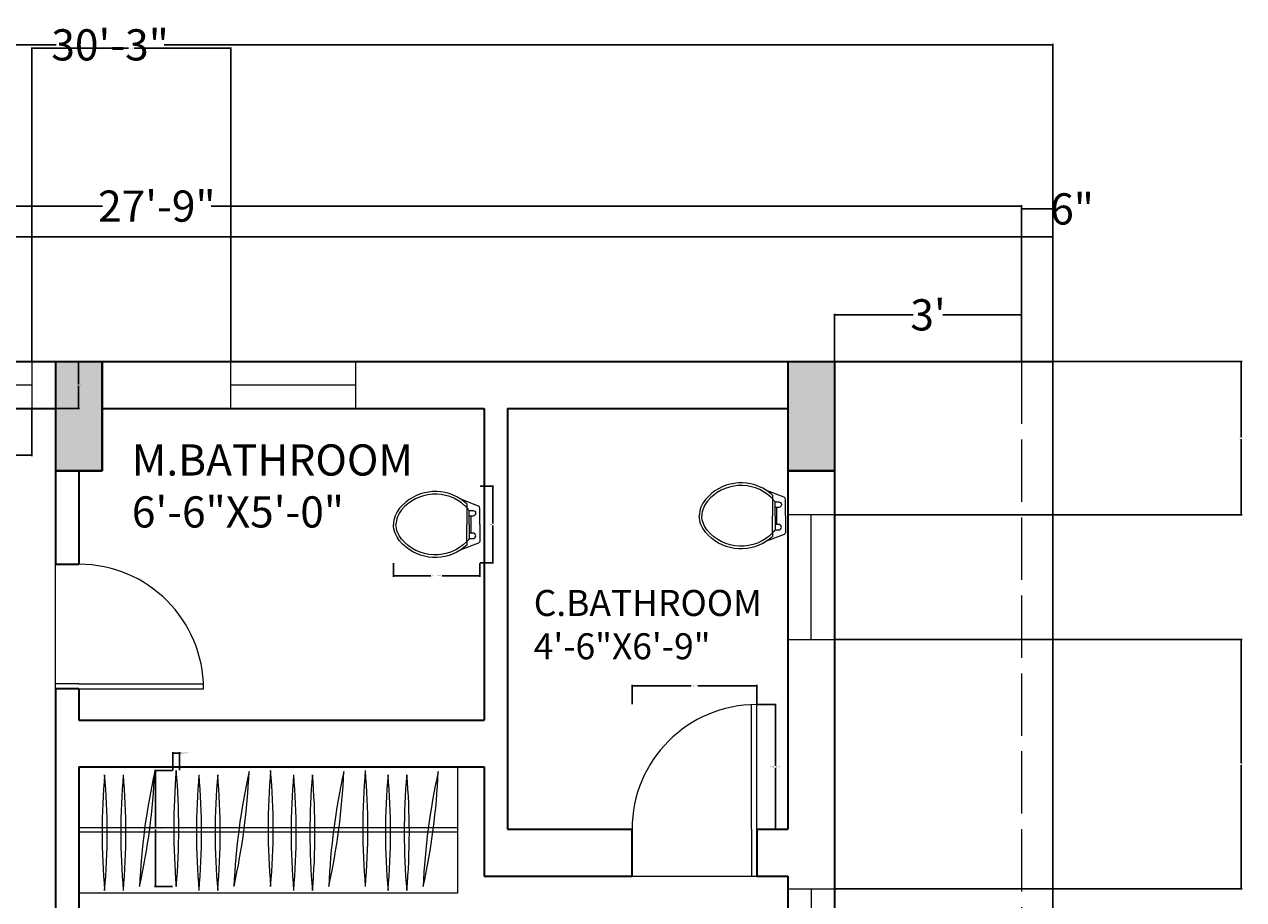
# Model space of a CAD drawing. Units: inches. Extents: x -36 to 401, y -686 to 73.
# Tile 15 of 15: x 167 to 401, y -96 to 73. Entities that reach past the tile are written whole.
import ezdxf

# ---------------------------------------------------------------- set-up
doc = ezdxf.new("R2010")
doc.units = ezdxf.units.IN
doc.header["$MEASUREMENT"] = 0
doc.linetypes.add('ACAD_ISO02W100', pattern=[15, 12, -3])
for name, color, linetype, lineweight in [('A-ANNO-DIMS', 2, 'Continuous', 18), ('A-AREA-IDEN', 7, 'Continuous', 18), ('A-COLS', 7, 'Continuous', 40), ('A-COLS-PATT', 22, 'Continuous', 13), ('A-DOOR', 3, 'Continuous', 18), ('A-FLOR-CASE', 9, 'Continuous', 18), ('A-FLOR-FIXT', 9, 'Continuous', 18), ('A-FLOR-OVHD', 8, 'ACAD_ISO02W100', 18), ('A-GLAZ', 4, 'Continuous', 18), ('A-WALL', 7, 'Continuous', 35), ('C-PROP', 7, 'Continuous', 25)]:
    doc.layers.add(name, color=color, linetype=linetype, lineweight=lineweight)
doc.styles.get("Standard").update_dxf_attribs({"font": 'arial.ttf'})
doc.dimstyles.get("Standard").update_dxf_attribs({"dimtxt": 0.18, "dimasz": 0.18, "dimexe": 0.18, "dimexo": 0.0625, "dimgap": 0.09, "dimtad": 0, "dimtih": 1, "dimtoh": 1, "dimdec": 0, "dimzin": 0, "dimdsep": 46, "dimlunit": 3, "dimtxsty": 'Standard', "dimcen": 0.09, "dimadec": 0, "dimazin": 0, "dimtfac": 1, "dimtdec": 0, "dimtofl": 0, "dimtmove": 0, "dimatfit": 3, "dimfxl": 1, "dimtolj": 1, "dimtzin": 0, "dimarcsym": 0})

# ---------------------------------------------------------------- blocks, each defined once
blk = doc.blocks.new('*D5')
at = {"layer": 'A-ANNO-DIMS', "color": 0, "lineweight": -2, "transparency": 16777216}
for p, q in [((25.69, 7.85), (25.69, 37.9)), ((25.87, 37.72), (181.74, 37.72)), ((358.51, 37.72), (202.64, 37.72)), ((358.69, 7.85), (358.69, 37.9))]:
    blk.add_line(p, q, dxfattribs=at)
at = {"layer": 'A-ANNO-DIMS', "color": 0, "transparency": 16777216}
for points in [[(25.87, 37.75), (25.87, 37.69), (25.69, 37.72)], [(358.51, 37.75), (358.51, 37.69), (358.69, 37.72)]]:
    blk.add_solid(points, dxfattribs=at)
at = {"layer": 'Defpoints', "color": 0, "transparency": 16777216}
for p in [(358.69, 37.72), (25.69, 7.79), (358.69, 7.79)]:
    blk.add_point(p, dxfattribs=at)
at = {"layer": 'A-ANNO-DIMS', "color": 0, "transparency": 16777216, "insert": (192.19, 37.72), "char_height": 6, "attachment_point": 5}
blk.add_mtext('\\A1;27\'-9"', dxfattribs=at)
blk = doc.blocks.new('*D6')
at = {"layer": 'A-ANNO-DIMS', "color": 0, "lineweight": -2, "transparency": 16777216}
for p, q in [((322.69, 7.85), (322.69, 16.97)), ((322.87, 16.79), (337.84, 16.79)), ((358.51, 16.79), (343.54, 16.79)), ((358.69, 7.85), (358.69, 16.97))]:
    blk.add_line(p, q, dxfattribs=at)
at = {"layer": 'A-ANNO-DIMS', "color": 0, "transparency": 16777216}
for points in [[(322.87, 16.82), (322.87, 16.76), (322.69, 16.79)], [(358.51, 16.82), (358.51, 16.76), (358.69, 16.79)]]:
    blk.add_solid(points, dxfattribs=at)
at = {"layer": 'Defpoints', "color": 0, "transparency": 16777216}
for p in [(358.69, 16.79), (322.69, 7.79), (358.69, 7.79)]:
    blk.add_point(p, dxfattribs=at)
at = {"layer": 'A-ANNO-DIMS', "color": 0, "transparency": 16777216, "insert": (340.69, 16.79), "char_height": 6, "attachment_point": 5}
blk.add_mtext("\\A1;3'", dxfattribs=at)
blk = doc.blocks.new('*D7')
at = {"layer": 'A-ANNO-DIMS', "color": 0, "lineweight": -2, "transparency": 16777216}
for p, q in [((358.69, 31.85), (358.69, 37.36)), ((358.87, 37.18), (364.51, 37.18)), ((364.69, 31.85), (364.69, 37.36)), ((364.69, 37.18), (364.87, 37.18))]:
    blk.add_line(p, q, dxfattribs=at)
at = {"layer": 'A-ANNO-DIMS', "color": 0, "transparency": 16777216}
for points in [[(358.87, 37.21), (358.87, 37.15), (358.69, 37.18)], [(364.51, 37.21), (364.51, 37.15), (364.69, 37.18)]]:
    blk.add_solid(points, dxfattribs=at)
at = {"layer": 'Defpoints', "color": 0, "transparency": 16777216}
for p in [(364.69, 37.18), (358.69, 31.79), (364.69, 31.79)]:
    blk.add_point(p, dxfattribs=at)
at = {"layer": 'A-ANNO-DIMS', "color": 0, "transparency": 16777216, "insert": (368.42, 37.18), "char_height": 6, "attachment_point": 5}
blk.add_mtext('\\A1;6"', dxfattribs=at)
blk = doc.blocks.new('*D9')
at = {"layer": 'A-ANNO-DIMS', "color": 0, "lineweight": -2, "transparency": 16777216}
for p, q in [((1.69, 31.85), (1.69, 68.93)), ((1.87, 68.75), (172.79, 68.75)), ((364.51, 68.75), (193.58, 68.75)), ((364.69, 31.85), (364.69, 68.93))]:
    blk.add_line(p, q, dxfattribs=at)
at = {"layer": 'A-ANNO-DIMS', "color": 0, "transparency": 16777216}
for points in [[(1.87, 68.78), (1.87, 68.72), (1.69, 68.75)], [(364.51, 68.78), (364.51, 68.72), (364.69, 68.75)]]:
    blk.add_solid(points, dxfattribs=at)
at = {"layer": 'Defpoints', "color": 0, "transparency": 16777216}
for p in [(364.69, 68.75), (1.69, 31.79), (364.69, 31.79)]:
    blk.add_point(p, dxfattribs=at)
at = {"layer": 'A-ANNO-DIMS', "color": 0, "transparency": 16777216, "insert": (183.19, 68.75), "char_height": 6, "attachment_point": 5}
blk.add_mtext('\\A1;30\'-3"', dxfattribs=at)
blk = doc.blocks.new('WIN-24IN')
for p, q in [((0, 9), (24, 9)), ((0, 0), (0, 9)), ((24, 9), (24, 0)), ((0, 4.5), (24, 4.5)), ((24, 0), (0, 0))]:
    blk.add_line(p, q)
blk = doc.blocks.new('WIN-60IN')
for p, q in [((0, 9), (60, 9)), ((0, 0), (0, 9)), ((60, 9), (60, 0)), ((0, 4.5), (60, 4.5)), ((60, 0), (0, 0))]:
    blk.add_line(p, q)
blk = doc.blocks.new('DOOR-SWING-24IN')
for p, q in [((0, 1), (24, 1)), ((0, 0), (24, 0))]:
    blk.add_line(p, q)
blk.add_arc((0, 0), 24, 0, 90)
blk = doc.blocks.new('WC-PLAN')
for p, q in [((14.11, 10.32), (14.11, 9.62)), ((14.11, 9.62), (14.11, 6.35)), ((14.11, 3.08), (14.11, 6.35)), ((14.11, 3.08), (14.11, 2.38))]:
    blk.add_line(p, q)
for points in [[(12.97, 11.22, 0.383919), (1.2, 9.48, 0.163732), (0, 6.35, 0.359733)], [(13.77, 9.96, 0.431639), (1.58, 9.16, 0.162618), (0.5, 6.35, 0.470877)], [(14.11, 10.32, 0.040937), (12.97, 11.22, 0.163732)], [(16.63, 6.35), (16.63, 9.53, 0.31031), (16.36, 9.92), (12.97, 11.22, 0.209071)], [(14.11, 9.62, 0.014165), (13.77, 9.96, 0.162618)], [(14.61, 9.05, 0.022712), (14.11, 9.62, 0.162618)], [(14.61, 6.35), (14.61, 9.05, 0.022712)], [(14.61, 9.05), (15.31, 9.05, -1), (15.31, 7.99), (14.95, 7.99)], [(12.97, 1.48, -0.383919), (1.2, 3.23, -0.163732), (0, 6.35, -0.359733)], [(14.11, 3.08, -0.448546), (1.58, 3.54, -0.162618), (0.5, 6.35, -0.470877)], [(16.63, 6.35), (16.63, 3.18, -0.31031), (16.36, 2.79), (12.97, 1.48, -0.209071)], [(14.61, 6.35), (14.61, 3.65, -0.476108)], [(14.61, 3.65), (15.31, 3.65, 1), (15.31, 4.72), (14.95, 4.72)], [(14.11, 2.38, -0.040937), (12.97, 1.48, -0.163732)], [(14.61, 3.65, -0.022712), (14.11, 3.08, -0.162618)]]:
    blk.add_lwpolyline(points, format="xyb")
for points in [[(14.95, 7.99), (14.61, 7.99)], [(14.95, 4.72), (14.95, 7.99)], [(14.95, 4.72), (14.61, 4.72)]]:
    blk.add_lwpolyline(points)
blk = doc.blocks.new('GARMENT-ON-RAIL-MEDIUM')
for centre, start, end in [((127.91, 11.14), 175.0028, 184.9972), ((-126.93, 11.14), 355.0028, 4.9972)]:
    blk.add_arc(centre, 127.91, start, end)
blk = doc.blocks.new('*D31')
at = {"layer": 'A-ANNO-DIMS', "color": 0, "lineweight": -2, "transparency": 16777216}
for p, q in [((195.21, -70.92), (191.75, -70.92)), ((191.93, -71.1), (191.93, -81.88)), ((191.93, -93.03), (191.93, -82.25)), ((195.21, -93.21), (191.75, -93.21))]:
    blk.add_line(p, q, dxfattribs=at)
at = {"layer": 'A-ANNO-DIMS', "color": 0, "transparency": 16777216}
for points in [[(191.9, -71.1), (191.96, -71.1), (191.93, -70.92)], [(191.9, -93.03), (191.96, -93.03), (191.93, -93.21)]]:
    blk.add_solid(points, dxfattribs=at)
at = {"layer": 'Defpoints', "color": 0, "transparency": 16777216}
for p in [(191.93, -70.92), (195.28, -70.92), (195.28, -93.21)]:
    blk.add_point(p, dxfattribs=at)
at = {"layer": 'A-ANNO-DIMS', "color": 0, "transparency": 16777216, "insert": (191.93, -82.07), "char_height": 0.18, "attachment_point": 5}
blk.add_mtext('\\A1;HANGER 1\'-10 1/2" TYP.', dxfattribs=at)
blk = doc.blocks.new('*D32')
at = {"layer": 'A-ANNO-DIMS', "color": 0, "lineweight": -2, "transparency": 16777216}
for p, q in [((195.28, -70.86), (195.28, -67.4)), ((195.46, -67.58), (196.39, -67.58)), ((196.57, -70.86), (196.57, -67.4)), ((196.57, -67.58), (196.75, -67.58))]:
    blk.add_line(p, q, dxfattribs=at)
at = {"layer": 'A-ANNO-DIMS', "color": 0, "transparency": 16777216}
for points in [[(195.46, -67.55), (195.46, -67.61), (195.28, -67.58)], [(196.39, -67.55), (196.39, -67.61), (196.57, -67.58)]]:
    blk.add_solid(points, dxfattribs=at)
at = {"layer": 'Defpoints', "color": 0, "transparency": 16777216}
for p in [(196.57, -67.58), (195.28, -70.92), (196.57, -70.92)]:
    blk.add_point(p, dxfattribs=at)
at = {"layer": 'A-ANNO-DIMS', "color": 0, "transparency": 16777216, "insert": (197.6, -67.58), "char_height": 0.18, "attachment_point": 5}
blk.add_mtext('\\A1;0\'-1 1/2" TYP.', dxfattribs=at)
blk = doc.blocks.new('*D37')
at = {"layer": 'A-ANNO-DIMS', "color": 0, "lineweight": -2, "transparency": 16777216}
for p, q in [((108.13, -1.27), (108.13, -10.39)), ((168.13, -1.27), (168.13, -10.39)), ((108.31, -10.21), (136.9, -10.21)), ((167.95, -10.21), (139.35, -10.21))]:
    blk.add_line(p, q, dxfattribs=at)
at = {"layer": 'A-ANNO-DIMS', "color": 0, "transparency": 16777216}
for points in [[(108.31, -10.18), (108.31, -10.24), (108.13, -10.21)], [(167.95, -10.18), (167.95, -10.24), (168.13, -10.21)]]:
    blk.add_solid(points, dxfattribs=at)
at = {"layer": 'Defpoints', "color": 0, "transparency": 16777216}
for p in [(108.13, -1.21), (168.13, -1.21), (168.13, -10.21)]:
    blk.add_point(p, dxfattribs=at)
at = {"layer": 'A-ANNO-DIMS', "color": 0, "transparency": 16777216, "insert": (138.13, -10.21), "char_height": 0.18, "attachment_point": 5}
blk.add_mtext('\\A1;WINDOW 5\'-0" TYP.', dxfattribs=at)
blk = doc.blocks.new('*D38')
at = {"layer": 'A-ANNO-DIMS', "color": 0, "lineweight": -2, "transparency": 16777216}
for p, q in [((168.19, 7.79), (177.31, 7.79)), ((177.13, 7.61), (177.13, 3.47)), ((177.13, -1.03), (177.13, 3.11)), ((168.19, -1.21), (177.31, -1.21))]:
    blk.add_line(p, q, dxfattribs=at)
at = {"layer": 'A-ANNO-DIMS', "color": 0, "transparency": 16777216}
for points in [[(177.1, 7.61), (177.16, 7.61), (177.13, 7.79)], [(177.1, -1.03), (177.16, -1.03), (177.13, -1.21)]]:
    blk.add_solid(points, dxfattribs=at)
at = {"layer": 'Defpoints', "color": 0, "transparency": 16777216}
for p in [(168.13, 7.79), (177.13, 7.79), (168.13, -1.21)]:
    blk.add_point(p, dxfattribs=at)
at = {"layer": 'A-ANNO-DIMS', "color": 0, "transparency": 16777216, "insert": (177.13, 3.29), "char_height": 0.18, "attachment_point": 5}
blk.add_mtext('\\A1;0\'-9" TYP.', dxfattribs=at)
blk = doc.blocks.new('*D43')
at = {"layer": 'A-ANNO-DIMS', "color": 0, "lineweight": -2, "transparency": 16777216}
for p, q in [((307.75, -58.21), (311.47, -58.21)), ((311.29, -58.39), (311.29, -70.03)), ((311.29, -82.03), (311.29, -70.39)), ((307.75, -82.21), (311.47, -82.21))]:
    blk.add_line(p, q, dxfattribs=at)
at = {"layer": 'A-ANNO-DIMS', "color": 0, "transparency": 16777216}
for points in [[(311.26, -58.39), (311.32, -58.39), (311.29, -58.21)], [(311.26, -82.03), (311.32, -82.03), (311.29, -82.21)]]:
    blk.add_solid(points, dxfattribs=at)
at = {"layer": 'Defpoints', "color": 0, "transparency": 16777216}
for p in [(307.69, -58.21), (311.29, -58.21), (307.69, -82.21)]:
    blk.add_point(p, dxfattribs=at)
at = {"layer": 'A-ANNO-DIMS', "color": 0, "transparency": 16777216, "insert": (311.29, -70.21), "char_height": 0.18, "attachment_point": 5}
blk.add_mtext('\\A1;DOOR 2\'-0" TYP.', dxfattribs=at)
blk = doc.blocks.new('*D44')
at = {"layer": 'A-ANNO-DIMS', "color": 0, "lineweight": -2, "transparency": 16777216}
for p, q in [((283.69, -58.15), (283.69, -54.43)), ((283.87, -54.61), (295.05, -54.61)), ((307.51, -54.61), (296.33, -54.61)), ((307.69, -58.15), (307.69, -54.43))]:
    blk.add_line(p, q, dxfattribs=at)
at = {"layer": 'A-ANNO-DIMS', "color": 0, "transparency": 16777216}
for points in [[(283.87, -54.58), (283.87, -54.64), (283.69, -54.61)], [(307.51, -54.58), (307.51, -54.64), (307.69, -54.61)]]:
    blk.add_solid(points, dxfattribs=at)
at = {"layer": 'Defpoints', "color": 0, "transparency": 16777216}
for p in [(283.69, -54.61), (283.69, -58.21), (307.69, -58.21)]:
    blk.add_point(p, dxfattribs=at)
at = {"layer": 'A-ANNO-DIMS', "color": 0, "transparency": 16777216, "insert": (295.69, -54.61), "char_height": 0.18, "attachment_point": 5}
blk.add_mtext('\\A1;2\'-0" TYP.', dxfattribs=at)
blk = doc.blocks.new('*D47')
at = {"layer": 'A-ANNO-DIMS', "color": 0, "lineweight": -2, "transparency": 16777216}
for p, q in [((237.74, -31.01), (237.74, -33.63)), ((254.37, -31.01), (254.37, -33.63)), ((237.92, -33.45), (244.96, -33.45)), ((254.19, -33.45), (247.15, -33.45))]:
    blk.add_line(p, q, dxfattribs=at)
at = {"layer": 'A-ANNO-DIMS', "color": 0, "transparency": 16777216}
for points in [[(237.92, -33.42), (237.92, -33.48), (237.74, -33.45)], [(254.19, -33.42), (254.19, -33.48), (254.37, -33.45)]]:
    blk.add_solid(points, dxfattribs=at)
at = {"layer": 'Defpoints', "color": 0, "transparency": 16777216}
for p in [(237.74, -30.95), (254.37, -30.95), (254.37, -33.45)]:
    blk.add_point(p, dxfattribs=at)
at = {"layer": 'A-ANNO-DIMS', "color": 0, "transparency": 16777216, "insert": (246.05, -33.45), "char_height": 0.18, "attachment_point": 5}
blk.add_mtext('\\A1;WC 1\'-4 1/2" TYP.', dxfattribs=at)
blk = doc.blocks.new('*D48')
at = {"layer": 'A-ANNO-DIMS', "color": 0, "lineweight": -2, "transparency": 16777216}
for p, q in [((254.43, -16.18), (257.04, -16.18)), ((256.86, -16.36), (256.86, -23.38)), ((256.86, -30.77), (256.86, -23.75)), ((254.43, -30.95), (257.04, -30.95))]:
    blk.add_line(p, q, dxfattribs=at)
at = {"layer": 'A-ANNO-DIMS', "color": 0, "transparency": 16777216}
for points in [[(256.83, -16.36), (256.89, -16.36), (256.86, -16.18)], [(256.83, -30.77), (256.89, -30.77), (256.86, -30.95)]]:
    blk.add_solid(points, dxfattribs=at)
at = {"layer": 'Defpoints', "color": 0, "transparency": 16777216}
for p in [(254.37, -16.18), (256.86, -16.18), (254.37, -30.95)]:
    blk.add_point(p, dxfattribs=at)
at = {"layer": 'A-ANNO-DIMS', "color": 0, "transparency": 16777216, "insert": (256.86, -23.56), "char_height": 0.18, "attachment_point": 5}
blk.add_mtext('\\A1;1\'-3" TYP.', dxfattribs=at)
blk = doc.blocks.new('*D67')
at = {"layer": 'A-ANNO-DIMS', "color": 0, "lineweight": -2, "transparency": 16777216}
for p, q in [((168.13, 7.85), (168.13, 68.27)), ((168.31, 68.09), (186.74, 68.09)), ((206.26, 68.09), (187.82, 68.09)), ((206.44, 7.85), (206.44, 68.27))]:
    blk.add_line(p, q, dxfattribs=at)
at = {"layer": 'A-ANNO-DIMS', "color": 0, "transparency": 16777216}
for points in [[(168.31, 68.12), (168.31, 68.06), (168.13, 68.09)], [(206.26, 68.12), (206.26, 68.06), (206.44, 68.09)]]:
    blk.add_solid(points, dxfattribs=at)
at = {"layer": 'Defpoints', "color": 0, "transparency": 16777216}
for p in [(206.44, 68.09), (168.13, 7.79), (206.44, 7.79)]:
    blk.add_point(p, dxfattribs=at)
at = {"layer": 'A-ANNO-DIMS', "color": 0, "transparency": 16777216, "insert": (187.28, 68.09), "char_height": 0.18, "attachment_point": 5}
blk.add_mtext('\\A1;3\'-2 1/2"', dxfattribs=at)
blk = doc.blocks.new('*D69')
at = {"layer": 'A-ANNO-DIMS', "color": 0, "lineweight": -2, "transparency": 16777216}
for p, q in [((322.75, 7.79), (401.17, 7.79)), ((400.99, 7.61), (400.99, -6.78)), ((400.99, -21.53), (400.99, -7.14)), ((322.75, -21.71), (401.17, -21.71))]:
    blk.add_line(p, q, dxfattribs=at)
at = {"layer": 'A-ANNO-DIMS', "color": 0, "transparency": 16777216}
for points in [[(400.96, 7.61), (401.02, 7.61), (400.99, 7.79)], [(400.96, -21.53), (401.02, -21.53), (400.99, -21.71)]]:
    blk.add_solid(points, dxfattribs=at)
at = {"layer": 'Defpoints', "color": 0, "transparency": 16777216}
for p in [(322.69, 7.79), (322.69, -21.71), (400.99, -21.71)]:
    blk.add_point(p, dxfattribs=at)
at = {"layer": 'A-ANNO-DIMS', "color": 0, "transparency": 16777216, "insert": (400.99, -6.96), "char_height": 0.18, "attachment_point": 5}
blk.add_mtext('\\A1;2\'-5 1/2"', dxfattribs=at)
blk = doc.blocks.new('*D70')
at = {"layer": 'A-ANNO-DIMS', "color": 0, "lineweight": -2, "transparency": 16777216}
for p, q in [((322.75, -45.71), (401.17, -45.71)), ((400.99, -45.89), (400.99, -69.51)), ((400.99, -93.5), (400.99, -69.87)), ((322.75, -93.68), (401.17, -93.68))]:
    blk.add_line(p, q, dxfattribs=at)
at = {"layer": 'A-ANNO-DIMS', "color": 0, "transparency": 16777216}
for points in [[(400.96, -45.89), (401.02, -45.89), (400.99, -45.71)], [(400.96, -93.5), (401.02, -93.5), (400.99, -93.68)]]:
    blk.add_solid(points, dxfattribs=at)
at = {"layer": 'Defpoints', "color": 0, "transparency": 16777216}
for p in [(322.69, -45.71), (322.69, -93.68), (400.99, -93.68)]:
    blk.add_point(p, dxfattribs=at)
at = {"layer": 'A-ANNO-DIMS', "color": 0, "transparency": 16777216, "insert": (400.99, -69.69), "char_height": 0.18, "attachment_point": 5}
blk.add_mtext('\\A1;4\'-0"', dxfattribs=at)

msp = doc.modelspace()

# ---------------------------------------------------------------- hatches: boundary and pattern name
at = {"layer": 'A-COLS-PATT'}
h = msp.add_hatch(color=256, dxfattribs=at)
h.dxf.hatch_style = 1
h.paths.add_polyline_path([(34.69, 7.79), (25.69, 7.79), (25.69, -13.21), (34.69, -13.21)])
h.paths.add_polyline_path([(172.69, -13.21), (177.19, -13.21), (181.69, -13.21), (181.69, 7.79), (172.69, 7.79)])
h.paths.add_polyline_path([(322.69, 7.79), (313.69, 7.79), (313.69, -13.21), (322.69, -13.21)])
h.paths.add_polyline_path([(322.69, -157.21), (313.69, -157.21), (313.69, -178.21), (322.69, -178.21)])
h.paths.add_polyline_path([(172.69, -178.21), (177.19, -178.21), (181.69, -178.21), (181.69, -157.21), (177.19, -157.21), (172.69, -157.21)])
h.paths.add_polyline_path([(25.69, -178.21), (34.69, -178.21), (34.69, -157.21), (25.69, -157.21)])
h.paths.add_polyline_path([(34.69, -325.21), (25.69, -325.21), (25.69, -346.21), (34.69, -346.21)])
h.paths.add_polyline_path([(181.69, -325.21), (177.19, -325.21), (172.69, -325.21), (172.69, -346.21), (177.19, -346.21), (181.69, -346.21)])
h.paths.add_polyline_path([(322.69, -325.21), (313.69, -325.21), (313.69, -346.21), (322.69, -346.21)])
h.paths.add_polyline_path([(364.69, -451.21), (358.69, -451.21), (358.69, -472.21), (364.69, -472.21)])
h.paths.add_polyline_path([(181.69, -451.21), (177.19, -451.21), (172.69, -451.21), (172.69, -472.21), (177.19, -472.21), (181.69, -472.21)])
h.paths.add_polyline_path([(25.69, -472.21), (34.69, -472.21), (34.69, -451.21), (25.69, -451.21)])

# ---------------------------------------------------------------- linework, layer by layer
at = {"layer": 'A-COLS'}
for p, q in [((181.69, -13.21), (181.69, 7.79)), ((177.19, -13.21), (172.69, -13.21)), ((177.19, -13.21), (181.69, -13.21)), ((313.69, -13.21), (322.69, -13.21))]:
    msp.add_line(p, q, dxfattribs=at)
at = {"layer": 'A-DOOR'}
for p, q in [((172.69, -55.21), (172.69, -31.21)), ((177.19, -54.21), (172.69, -54.21)), ((306.69, -82.21), (306.69, -91.21)), ((283.69, -91.21), (307.69, -91.21))]:
    msp.add_line(p, q, dxfattribs=at)
at = {"layer": 'A-FLOR-CASE'}
for p, q in [((250.11, -70.21), (177.19, -70.21)), ((177.19, -70.21), (177.19, -94.52)), ((250.11, -70.21), (250.11, -94.52)), ((250.11, -81.96), (177.19, -81.96)), ((250.11, -82.77), (177.19, -82.77)), ((250.11, -94.52), (177.19, -94.52))]:
    msp.add_line(p, q, dxfattribs=at)
at = {"layer": 'A-FLOR-OVHD'}
msp.add_line((358.69, 7.79), (358.69, -559.77), dxfattribs=at)
at = {"layer": 'A-WALL'}
for p, q in [((25.69, 7.79), (364.69, 7.79)), ((172.69, 7.79), (172.69, -31.21)), ((313.69, 7.79), (313.69, -82.21)), ((322.69, 7.79), (322.69, -271.21)), ((34.69, -1.21), (172.69, -1.21)), ((181.69, -1.21), (255.19, -1.21)), ((255.19, -1.21), (255.19, -61.21)), ((259.69, -1.21), (259.69, -82.21)), ((259.69, -1.21), (313.69, -1.21)), ((177.19, -13.21), (177.19, -31.21)), ((172.69, -31.21), (177.19, -31.21)), ((177.19, -55.21), (172.69, -55.21)), ((172.69, -55.21), (172.69, -181.21)), ((177.19, -55.21), (177.19, -61.21)), ((177.19, -61.21), (255.19, -61.21)), ((177.19, -70.21), (255.19, -70.21)), ((177.19, -70.21), (177.19, -157.21)), ((255.19, -70.21), (255.19, -91.21)), ((259.69, -82.21), (283.69, -82.21)), ((283.69, -91.21), (283.69, -82.21)), ((307.69, -82.21), (307.69, -91.21)), ((307.69, -82.21), (313.69, -82.21)), ((255.19, -91.21), (283.69, -91.21)), ((307.69, -91.21), (313.69, -91.21)), ((313.69, -91.21), (313.69, -223.21))]:
    msp.add_line(p, q, dxfattribs=at)
at = {"layer": 'C-PROP'}
for p, q in [((1.69, 31.79), (364.69, 31.79)), ((364.69, 31.79), (364.69, -649.21))]:
    msp.add_line(p, q, dxfattribs=at)

# ---------------------------------------------------------------- block references
at = {"layer": 'A-DOOR'}
msp.add_blockref('DOOR-SWING-24IN', (177.19, -55.21), dxfattribs=at)
at = {"layer": 'A-DOOR', "rotation": 90}
msp.add_blockref('DOOR-SWING-24IN', (307.69, -82.21), dxfattribs=at)
at = {"layer": 'A-FLOR-CASE'}
for p in [(181.65, -93.99), (185.25, -93.99), (195.44, -93.21), (199.82, -93.99), (203.42, -93.99), (213.61, -93.21), (218.05, -93.99), (221.66, -93.99), (231.85, -93.21), (236.22, -93.99), (239.83, -93.99)]:
    msp.add_blockref('GARMENT-ON-RAIL-MEDIUM', p, dxfattribs=at)
for p, rotation in [((192.27, -71.18), 172.5051423894902), ((210.44, -71.18), 172.5051423894902), ((224.81, -93.15), 352.5051423895286), ((242.98, -93.15), 352.5051423896668)]:
    msp.add_blockref('GARMENT-ON-RAIL-MEDIUM', p, dxfattribs=dict(at, rotation=rotation))
at = {"layer": 'A-FLOR-FIXT'}
for p in [(237.74, -29.92), (296.62, -28.25)]:
    msp.add_blockref('WC-PLAN', p, dxfattribs=at)
at = {"layer": 'A-GLAZ'}
for name, p in [('WIN-60IN', (108.12, -1.21)), ('WIN-24IN', (206.44, -1.21))]:
    msp.add_blockref(name, p, dxfattribs=at)
at = {"layer": 'A-GLAZ', "extrusion": (0, 0, -1), "zscale": -1, "rotation": 90}
msp.add_blockref('WIN-24IN', (-313.69, -45.71), dxfattribs=at)
at = {"layer": 'A-GLAZ', "rotation": 270}
msp.add_blockref('WIN-60IN', (313.69, -93.68), dxfattribs=at)

# ---------------------------------------------------------------- texts
at = {"layer": 'A-AREA-IDEN', "attachment_point": 1}
for s, insert, char_height in [('M.BATHROOM\\P6\'-6"X5\'-0"', (187.38, -8.14), 6), ('C.BATHROOM\\P4\'-6"X6\'-9"', (264.76, -36.16), 5)]:
    msp.add_mtext(s, dxfattribs=dict(at, insert=insert, char_height=char_height))

# ---------------------------------------------------------------- dimensions: what is measured, and where the dimension line sits
at = {"layer": 'A-ANNO-DIMS'}
for base, p1, p2, override, picture, middle in [((364.69, 68.75), (1.69, 31.79), (364.69, 31.79), {"dimtxt": 6, "dimclrd": 0, "dimclre": 0, "dimclrt": 0}, '*D9', (183.19, 68.75)), ((206.44, 68.09), (168.13, 7.79), (206.44, 7.79), {"dimdec": 1, "dimlfac": 1, "dimrnd": 0, "dimzin": 1, "dimdsep": 46, "dimlunit": 4, "dimfrac": 2}, '*D67', (187.28, 68.09)), ((358.69, 37.72), (25.69, 7.79), (358.69, 7.79), {"dimtxt": 6, "dimclrd": 0, "dimclre": 0, "dimclrt": 0}, '*D5', (192.19, 37.72)), ((364.69, 37.18), (358.69, 31.79), (364.69, 31.79), {"dimtxt": 6, "dimclrd": 0, "dimclre": 0, "dimclrt": 0}, '*D7', (368.42, 37.18)), ((358.69, 16.79), (322.69, 7.79), (358.69, 7.79), {"dimtxt": 6, "dimclrd": 0, "dimclre": 0, "dimclrt": 0}, '*D6', (340.69, 16.79))]:
    dim = msp.add_linear_dim(base=base, p1=p1, p2=p2, dimstyle='Standard', override=override, dxfattribs=at)
    dim.commit()
    dim.dimension.update_dxf_attribs({"geometry": picture, "text_midpoint": middle})
for base, p1, p2, angle, text, picture, middle in [((177.13, 7.79), (168.13, -1.21), (168.13, 7.79), 90, '<> TYP.', '*D38', (177.13, 3.29)), ((256.86, -16.18), (254.37, -30.95), (254.37, -16.18), 90, '<> TYP.', '*D48', (256.86, -23.56)), ((283.69, -54.61), (307.69, -58.21), (283.69, -58.21), 180, '<> TYP.', '*D44', (295.69, -54.61)), ((311.29, -58.21), (307.69, -82.21), (307.69, -58.21), 90, 'DOOR <> TYP.', '*D43', (311.29, -70.21)), ((191.93, -70.92), (195.28, -93.21), (195.28, -70.92), 90, 'HANGER <> TYP.', '*D31', (191.93, -82.07))]:
    dim = msp.add_linear_dim(base=base, p1=p1, p2=p2, angle=angle, text=text, dimstyle='Standard', override={"dimdec": 1, "dimlfac": 1, "dimrnd": 0, "dimzin": 1, "dimdsep": 46, "dimlunit": 4, "dimfrac": 2}, dxfattribs=at)
    dim.commit()
    dim.dimension.update_dxf_attribs({"geometry": picture, "text_midpoint": middle})
for base, p1, p2, picture, middle in [((400.99, -21.71), (322.69, 7.79), (322.69, -21.71), '*D69', (400.99, -6.96)), ((400.99, -93.68), (322.69, -45.71), (322.69, -93.68), '*D70', (400.99, -69.69))]:
    dim = msp.add_linear_dim(base=base, p1=p1, p2=p2, angle=90, dimstyle='Standard', override={"dimdec": 1, "dimlfac": 1, "dimrnd": 0, "dimzin": 1, "dimdsep": 46, "dimlunit": 4, "dimfrac": 2}, dxfattribs=at)
    dim.commit()
    dim.dimension.update_dxf_attribs({"geometry": picture, "text_midpoint": middle})
for base, p1, p2, text, picture, middle in [((168.13, -10.21), (108.13, -1.21), (168.13, -1.21), 'WINDOW <> TYP.', '*D37', (138.13, -10.21)), ((254.37, -33.45), (237.74, -30.95), (254.37, -30.95), 'WC <> TYP.', '*D47', (246.05, -33.45)), ((196.57, -67.58), (195.28, -70.92), (196.57, -70.92), '<> TYP.', '*D32', (197.6, -67.58))]:
    dim = msp.add_linear_dim(base=base, p1=p1, p2=p2, text=text, dimstyle='Standard', override={"dimdec": 1, "dimlfac": 1, "dimrnd": 0, "dimzin": 1, "dimdsep": 46, "dimlunit": 4, "dimfrac": 2}, dxfattribs=at)
    dim.commit()
    dim.dimension.update_dxf_attribs({"geometry": picture, "text_midpoint": middle})

doc.saveas('drawing.dxf')
